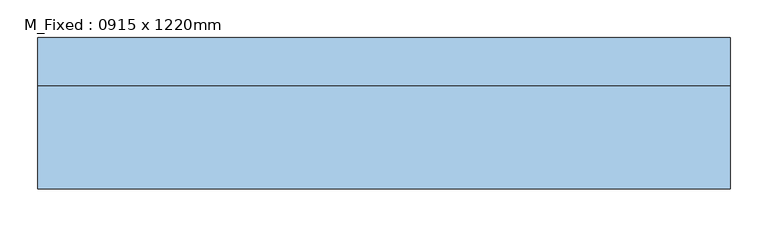
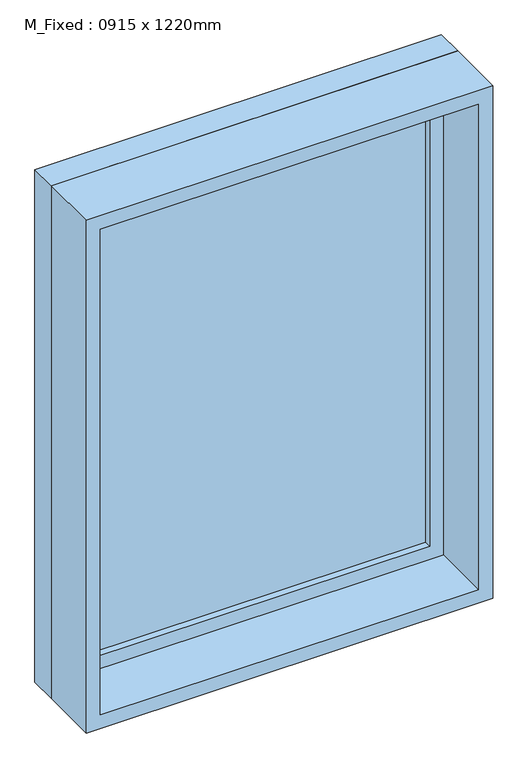
"""IFC4 building model written with IfcOpenShell, lengths in millimetres: window geometry, M_Fixed : 0915 x 1220mm."""

from ifc_helpers import new_model, si_unit, frame, origin, place, context, project, spatial, polyline, outline, extrude, source, transform, mapped, element, save


def m_fixed_0915_x_1220mm_488fb2fb(model_context):
    return source(origin(), model_context, "Body", "SweptSolid", [
        extrude(outline(polyline([(-394.5, 78.0), (394.5, 78.0), (394.5, 66.0), (-394.5, 66.0), (-394.5, 78.0)])), frame((0.0, 0.0, 978.0), z_axis=(0.0, 0.0, 1.0), x_axis=(1.0, 0.0, 0.0)), (0.0, 0.0, 1.0), 1094.0),
        extrude(outline(polyline([(2116.0, -438.5), (934.0, -438.5), (934.0, 438.5), (2116.0, 438.5), (2116.0, -438.5)]), holes=[polyline([(2072.0, -394.5), (2072.0, 394.5), (978.0, 394.5), (978.0, -394.5), (2072.0, -394.5)])]), frame((0.0, 50.0, 0.0), z_axis=(0.0, 1.0, 0.0), x_axis=(0.0, 0.0, 1.0)), (0.0, 0.0, 1.0), 44.0),
        extrude(outline(polyline([(2135.0, -457.5), (915.0, -457.5), (915.0, 457.5), (2135.0, 457.5), (2135.0, -457.5)]), holes=[polyline([(2116.0, -438.5), (2116.0, 438.5), (934.0, 438.5), (934.0, -438.5), (2116.0, -438.5)])]), frame((0.0, 50.0, 0.0), z_axis=(0.0, 1.0, 0.0), x_axis=(0.0, 0.0, 1.0)), (0.0, 0.0, 1.0), 63.0),
        extrude(outline(polyline([(2135.0, -457.5), (915.0, -457.5), (915.0, 457.5), (2135.0, 457.5), (2135.0, -457.5)]), holes=[polyline([(2103.0, -425.5), (2103.0, 425.5), (947.0, 425.5), (947.0, -425.5), (2103.0, -425.5)])]), frame((0.0, -87.0, 0.0), z_axis=(0.0, 1.0, 0.0), x_axis=(0.0, 0.0, 1.0)), (0.0, 0.0, 1.0), 137.0),
    ])


if __name__ == "__main__":
    model = new_model("IFC4")
    model_context = context("Model", 3, world=origin())
    ifc_project = project(units=[si_unit("LENGTHUNIT", "METRE", prefix="MILLI")], contexts=[model_context])
    site = spatial("IfcSite", under=ifc_project)
    building = spatial("IfcBuilding", under=site)
    placement = place(None, origin())
    m_fixed_0915_x_1220mm_shape = m_fixed_0915_x_1220mm_488fb2fb(model_context)
    element("IfcWindow", 1, ObjectType="M_Fixed : 0915 x 1220mm", at=placement, inside=building, context=model_context, shape_type="MappedRepresentation", body=[
        mapped(m_fixed_0915_x_1220mm_shape, transform((0.0, 0.0, 0.0), x_axis=(1.0, 0.0, 0.0), y_axis=(0.0, 1.0, 0.0), z_axis=(0.0, 0.0, 1.0))),
    ])
    save(model, "model.ifc")

# Revit data of these elements
# Type "M_Fixed : 0915 x 1220mm"
#   Type Mark = "15"
#   Height = 1220 mm
#   Default Sill Height = 915 mm
#   Width = 915 mm
#   Window Inset = 19 mm
#   Frame Exterior Material = Sash
#   Frame Interior Material = Sash
#   Glass Pane Material = Glass
#   Sash = Sash
#   Wall Closure = (empty or 0)
# Element 1 (IfcWindow, "M_Fixed : 0915 x 1220mm")
#   Materials on its faces: "Sash", "Glass"
# Materials
#   "Sash": class "Wood", colour RGB 136 99 55, transparency 0
#   "Glass": class "Glass", colour RGB 218 227 224, transparency 0.85, Description = "Soda Lime Glass", Cost = 0
